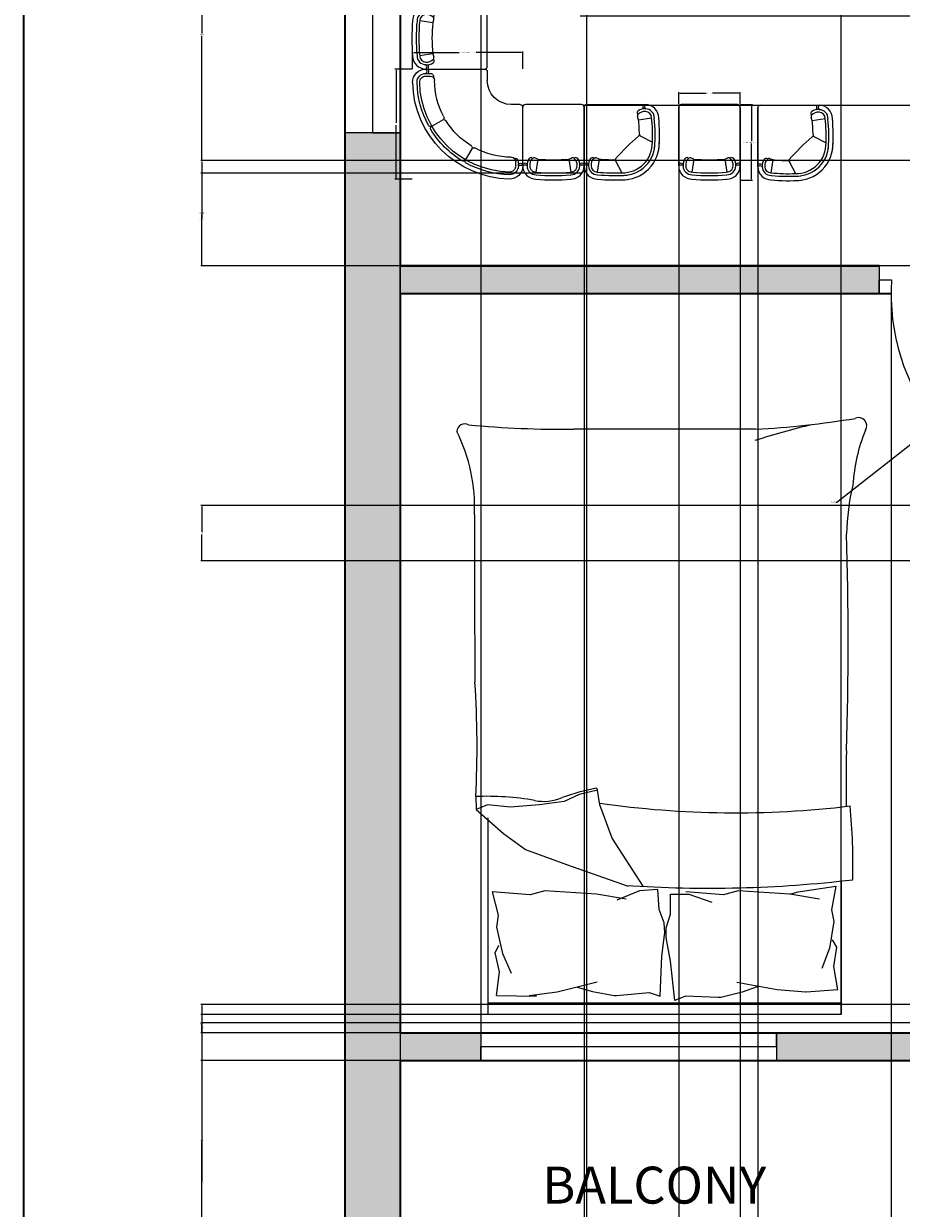
# Model space of a CAD drawing. Units: inches. Extents: x 2606 to 3027, y 1906 to 2463.
# Tile 2 of 10: x 2606 to 2748, y 2004 to 2196. Entities that reach past the tile are written whole.
import ezdxf

# ---------------------------------------------------------------- set-up
doc = ezdxf.new("R2010")
doc.units = ezdxf.units.IN
for name, color, linetype, lineweight in [('A-ANNO-DIMS', 2, 'Continuous', 18), ('A-ANNO-TTLB', 7, 'Continuous', 35), ('A-AREA-IDEN', 7, 'Continuous', 18), ('A-DOOR', 3, 'Continuous', 18), ('A-FURN', 8, 'Continuous', 13), ('A-GLAZ', 4, 'Continuous', 18), ('A-WALL', 7, 'Continuous', 35)]:
    doc.layers.add(name, color=color, linetype=linetype, lineweight=lineweight)
doc.layers.add('A-WALL-PATT', color=251, linetype='Continuous', lineweight=13, true_color=0x636466)
doc.styles.get("Standard").update_dxf_attribs({"font": 'arial.ttf'})
doc.dimstyles.get("Standard").update_dxf_attribs({"dimtxt": 0.18, "dimasz": 0.18, "dimexe": 0.18, "dimexo": 0.0625, "dimgap": 0.09, "dimtad": 0, "dimtih": 1, "dimtoh": 1, "dimdec": 4, "dimzin": 0, "dimdsep": 46, "dimtxsty": 'Standard', "dimcen": 0.09, "dimadec": 0, "dimazin": 0, "dimtfac": 1, "dimtdec": 4, "dimtofl": 0, "dimtmove": 0, "dimatfit": 3, "dimfxl": 1, "dimtolj": 1, "dimtzin": 0, "dimarcsym": 0})

# ---------------------------------------------------------------- blocks, each defined once
blk = doc.blocks.new('A$C707258B2')
at = {"color": 0}
for p, q in [((0.404, 0.342), (1.074, 0.342)), ((0.404, 0.292), (0.454, 0.292)), ((1.104, 0.312), (1.104, 0.212)), ((0.404, 0.262), (0.454, 0.262)), ((1.479, -0.063), (1.379, -0.063)), ((1.509, -0.763), (1.509, -0.093)), ((0.6, -0.238), (0.47, -0.313)), ((0.929, -0.567), (0.854, -0.697)), ((1.429, -0.763), (1.429, -0.713)), ((1.459, -0.763), (1.459, -0.712))]:
    blk.add_line(p, q, dxfattribs=at)
for centre, radius, start, end in [((0.404, 0.192), 0.15, 90, 181.1754), ((0.404, 0.192), 0.1, 90, 181.1754), ((0.378, 0.317), 0.0362, 316.3972, 43.6028), ((0.368, 0.317), 0.0662, 337.8298, 22.1702), ((0.455, 0.256), 0.0357, 345.4262, 90.5555), ((1.074, 0.312), 0.03, 360, 90), ((1.379, 0.212), 1.125, 181.1754, 268.8246), ((1.379, 0.212), 1.075, 181.1754, 208.6357), ((0.404, 0.192), 0.07, 90, 181.1754), ((1.379, 0.212), 1.045, 181.1754, 268.8246), ((0.454, 0.212), 0.05, 360, 90), ((1.379, 0.212), 0.875, 180, 208.4082), ((1.379, 0.212), 0.275, 180, 270), ((1.479, -0.093), 0.03, 360, 90), ((0.587, -0.216), 0.025, 300, 28.4082), ((0.612, -0.259), 0.025, 31.5918, 120), ((1.379, 0.212), 0.875, 211.5918, 238.4082), ((0.457, -0.291), 0.025, 208.6357, 300), ((0.482, -0.334), 0.025, 120, 211.3643), ((1.379, 0.212), 1.075, 211.3643, 238.6357), ((0.907, -0.555), 0.025, 330, 58.4082), ((0.951, -0.58), 0.025, 61.5918, 150), ((1.379, 0.212), 0.875, 241.5918, 270), ((1.379, -0.713), 0.05, 360, 90), ((0.832, -0.685), 0.025, 238.6357, 330), ((0.876, -0.71), 0.025, 150, 241.3643), ((1.379, 0.212), 1.075, 241.3643, 268.8246), ((1.359, -0.763), 0.15, 268.8246, 360), ((1.359, -0.763), 0.1, 268.8246, 360), ((1.359, -0.763), 0.07, 268.8246, 360), ((1.425, -0.709), 0.0336, 354.6301, 109.3883), ((1.484, -0.799), 0.0662, 67.8298, 112.1702), ((1.484, -0.789), 0.0362, 46.3972, 133.6028)]:
    blk.add_arc(centre, radius, start, end, dxfattribs=at)
blk = doc.blocks.new('part 01')
at = {"color": 0}
for p, q in [((-670, 700), (0, 700)), ((-591, 527), (-740, 550)), ((-591, 527), (-579, 561)), ((30, 30), (30, 670)), ((-591, 173), (-740, 150)), ((-591, 173), (-579, 139)), ((-670, 0), (0, 0))]:
    blk.add_line(p, q, dxfattribs=at)
for centre, radius, start, end in [((-670, 550), 150, 90, 181.1754), ((-696, 675), 36.2, 316.3972, 43.6028), ((-706, 675), 66.2, 337.8298, 22.1702), ((0, 670), 30, 0, 90), ((1178, 350), 2008, 174.2835, 185.7165), ((1178, 350), 1958, 174.2835, 185.7165), ((-670, 550), 100, 90, 181.1754), ((1178, 350), 1928, 174.2835, 185.7165), ((-670, 550), 70, 90, 181.1754), ((-660, 518), 133, 56.0897, 95.6132), ((-660, 518), 103, 42.0066, 95.6132), ((-600, 607), 25, 332.9608, 56.0897), ((-625, 620), 53.2, 321.0017, 332.9608), ((-602, 570), 25, 340, 42.0066), ((1178, 350), 1778, 174.2835, 185.7165), ((-670, 150), 150, 178.8246, 270), ((-670, 150), 100, 178.8246, 270), ((-670, 150), 70, 178.8246, 270), ((-602, 130), 25, 317.9934, 20), ((-660, 182), 133, 264.3868, 303.9103), ((-660, 182), 103, 264.3868, 317.9934), ((-696, 25), 36.2, 316.3972, 43.6028), ((-706, 25), 66.2, 337.8298, 22.1702), ((-600, 93), 25, 303.9103, 27.0392), ((-625, 80), 53.2, 27.0392, 38.9983), ((0, 30), 30, 270, 0)]:
    blk.add_arc(centre, radius, start, end, dxfattribs=at)
blk = doc.blocks.new('part02')
at = {"color": 0}
for p, q in [((0, -670), (0, 0)), ((30, 30), (700, 30)), ((621, -143), (609, -109)), ((621, -143), (770, -120)), ((640, -326), (778, -399)), ((173, -591), (139, -579)), ((173, -591), (150, -740)), ((356, -610), (429, -748))]:
    blk.add_line(p, q, dxfattribs=at)
for centre, radius, start, end in [((30, 0), 30, 90, 180), ((726, 5), 56.2, 153.6122, 206.6666), ((726, 5), 36.2, 136.3972, 223.6028), ((700, -120), 150, 0, 90), ((630, -63), 25, 123.9103, 207.0392), ((655, -50), 53.2, 207.0392, 218.9983), ((632, -100), 25, 137.9934, 200), ((690, -152), 103, 84.3868, 137.9934), ((689, -151), 132, 85.4378, 123.9887), ((700, -121), 101, 357.5006, 89.858), ((700, -120), 70, 0, 90), ((-1228, -320), 2008, 357.7349, 5.7032), ((-1148, -320), 1958, 355.8657, 5.7165), ((-1148, -320), 2008, 355.818, 5.7165), ((-1148, -320), 1778, 0.3836, 5.7165), ((2220, -2190), 2454, 130.6961, 139.3039), ((439, -409), 419, 268.2181, 1.7819), ((439, -409), 369, 268.2181, 1.7819), ((439, -409), 339, 268.2181, 1.7819), ((632, -344), 20, 62, 130.6961), ((650, -308), 20, 180.3836, 242), ((25, -696), 56.2, 63.3334, 116.3878), ((25, -696), 36.2, 46.3972, 133.6028), ((150, -670), 150, 180, 271.1754), ((182, -660), 133, 146.0897, 185.6132), ((150, -670), 100, 180, 271.1754), ((93, -600), 25, 62.9608, 146.0897), ((182, -660), 103, 132.0066, 185.6132), ((150, -670), 70, 180, 270), ((80, -625), 53.2, 51.0017, 62.9608), ((130, -602), 25, 70, 132.0066), ((350, 1178), 1778, 264.2835, 269.6164), ((338, -620), 20, 28, 89.6164), ((374, -602), 20, 139.3039, 208), ((350, 1258), 2008, 264.2968, 272.2651), ((350, 1178), 1958, 264.2835, 274.1343), ((350, 1178), 2008, 264.2835, 274.182)]:
    blk.add_arc(centre, radius, start, end, dxfattribs=at)
blk = doc.blocks.new('BED-DOUBLE')
for p, q in [((4.17, 75.16), (4.17, 96.87)), ((4.17, 96.87), (61.46, 96.87)), ((61.46, 96.87), (61.46, 64.97)), ((4.17, 95.03), (61.46, 95.03)), ((29.42, 93.94), (31.15, 94.63)), ((31.15, 94.63), (31.84, 88.22)), ((4.67, 92.87), (9.81, 93.27)), ((4.67, 92.9), (5.36, 89.08)), ((9.81, 93.27), (9.93, 93.24)), ((9.93, 93.24), (14.52, 92.9)), ((14.52, 92.9), (21.1, 91.68)), ((17.81, 92.38), (20.24, 93.24)), ((20.24, 93.24), (23.7, 94.11)), ((23.7, 94.11), (24.09, 94.11)), ((24.09, 94.11), (29.42, 93.94)), ((33.54, 93.89), (33.25, 87.44)), ((35.31, 93.3), (33.54, 93.89)), ((40.62, 93.81), (35.31, 93.3)), ((41.01, 93.83), (40.62, 93.81)), ((44.52, 93.18), (41.01, 93.83)), ((50.25, 93.19), (43.75, 91.57)), ((47, 92.47), (44.52, 93.18)), ((54.8, 93.82), (50.25, 93.19)), ((60.08, 93.81), (53.6, 93.92)), ((53.6, 93.92), (54.8, 93.82)), ((60.08, 93.81), (59.62, 89.96)), ((5.36, 89.08), (4.84, 85.96)), ((6.06, 86.14), (7.27, 89.43)), ((59.12, 86.97), (57.7, 90.18)), ((59.62, 89.96), (60.34, 86.88)), ((31.84, 88.22), (32.54, 84.4)), ((33.25, 87.44), (32.79, 83.59)), ((60.08, 82.69), (59.12, 86.97)), ((60.34, 86.88), (59.72, 85.62)), ((4.84, 85.96), (5.54, 84.75)), ((5.36, 81.8), (6.06, 86.14)), ((32.54, 82.84), (31.84, 80.59)), ((32.54, 84.4), (32.54, 82.84)), ((32.79, 83.59), (32.89, 82.03)), ((5.71, 79.9), (5.36, 81.8)), ((32.89, 82.03), (33.72, 79.83)), ((59.85, 80.77), (60.08, 82.69)), ((5.02, 76.08), (5.71, 79.9)), ((31.84, 80.59), (31.84, 77.38)), ((33.72, 79.83), (33.92, 76.62)), ((60.78, 77), (59.85, 80.77)), ((11.13, 76.95), (5.02, 76.08)), ((7.65, 78.14), (12.48, 77.34)), ((12.48, 77.34), (11.13, 76.95)), ((12.48, 77.34), (20.89, 76.82)), ((20.89, 76.82), (23.24, 77.49)), ((23.24, 77.49), (29.39, 77)), ((28.9, 77.38), (25.13, 78.68)), ((31.84, 77.38), (28.9, 77.38)), ((36.87, 76.8), (40.55, 78.34)), ((39.04, 78.14), (43.87, 77.34)), ((43.87, 77.34), (52.28, 76.82)), ((52.28, 76.82), (54.63, 77.49)), ((54.63, 77.49), (60.78, 77)), ((33.92, 76.62), (36.87, 76.8)), ((36.28, 76.03), (41.3, 68.25)), ((48.73, 72.52), (38.73, 76.03)), ((55.41, 70.1), (48.73, 72.52)), ((58.94, 67.51), (55.41, 70.1)), ((41.3, 68.25), (43.34, 62.87)), ((63.38, 63.61), (58.94, 67.51)), ((61.54, 62.87), (63.38, 63.61)), ((63.48, 61.52), (63.38, 63.61, 4.64)), ((43.34, 62.87), (43.71, 60.45)), ((46.68, 61.2), (49.1, 62.31)), ((49.1, 62.31), (53.18, 62.87)), ((53.18, 62.87), (57.82, 63.24)), ((57.82, 63.24), (61.54, 62.87)), ((43.71, 60.45), (46.68, 61.2)), ((18.06, 1.87), (47.57, 1.87))]:
    blk.add_line(p, q)
for centre, radius, start, end in [((102.1, 72.78), 99.87, 178.7218, 185.604), ((25.61, -121.38), 197.77, 86.0865, 96.7821), ((21.29, -90.53), 154.68, 81.7845, 96.9006), ((-200.58, 59.5), 203.94, 358.4762, 1.0082), ((37.35, 95.1), 35.55, 280.6617, 289.8806), ((52.44, 54.83), 7.46, 78.6608, 113.7384), ((61.53, 104.85), 43.38, 259.8763, 272.5657), ((43.92, 60.38), 0.221, 160.2464, 271.1377), ((218.51, 53.34), 155.25, 176.9791, 183.8365), ((581.23, 36.19), 578.22, 178.22771, 181.71854), ((-5405.34, 15.56), 5469.02, 0.00217, 0.28689), ((-32.25, 19.53), 35.53, 346.0648, 358.9113), ((91.3, 14.55), 27.65, 177.4714, 206.4681), ((-25.97, 12.62), 28.25, 337.9751, 356.652), ((1.3, 1.3), 1.31, 146.1736, 293.4781), ((-20.65, 125.3), 127.63, 283.3832, 287.7053), ((65.23, 2.32), 1.32, 242.6588, 356.02), ((25.69, -143.9), 145.97, 92.9958, 99.4091), ((49.34, -157.62), 159.5, 84.4998, 90.6351)]:
    blk.add_arc(centre, radius, start, end)
blk = doc.blocks.new('WIN-60IN')
for p, q in [((0, 9), (0, 0)), ((60, 4.5), (60, 9)), ((60, 9), (60, 0)), ((0, 0), (0, 4.5)), ((0, 4.5), (60, 4.5))]:
    blk.add_line(p, q)
blk = doc.blocks.new('WIN-48IN')
for p, q in [((0, 4.5), (0, 0)), ((48, 2.25), (48, 4.5)), ((48, 4.5), (48, 0)), ((0, 0), (0, 2.25)), ((0, 2.25), (48, 2.25))]:
    blk.add_line(p, q)
blk = doc.blocks.new('*D17')
at = {"layer": 'A-ANNO-DIMS', "color": 0, "lineweight": -2, "transparency": 16777216}
for p, q in [((2722.29, 2183.31), (2724.25, 2183.31)), ((2724.07, 2183.13), (2724.07, 2177.34)), ((2724.07, 2171.2), (2724.07, 2176.98)), ((2722.29, 2171.02), (2724.25, 2171.02))]:
    blk.add_line(p, q, dxfattribs=at)
at = {"layer": 'A-ANNO-DIMS', "color": 0, "transparency": 16777216}
for points in [[(2724.04, 2183.13), (2724.1, 2183.13), (2724.07, 2183.31)], [(2724.04, 2171.2), (2724.1, 2171.2), (2724.07, 2171.02)]]:
    blk.add_solid(points, dxfattribs=at)
at = {"layer": 'Defpoints', "color": 0, "transparency": 16777216}
for p in [(2722.23, 2183.31), (2724.07, 2183.31), (2722.23, 2171.02)]:
    blk.add_point(p, dxfattribs=at)
at = {"layer": 'A-ANNO-DIMS', "color": 0, "transparency": 16777216, "insert": (2724.07, 2177.16), "char_height": 0.18, "attachment_point": 5}
blk.add_mtext('\\A1;SEAT MODULE 12 TYP.', dxfattribs=at)
blk = doc.blocks.new('*D18')
at = {"layer": 'A-ANNO-DIMS', "color": 0, "lineweight": -2, "transparency": 16777216}
for p, q in [((2712.26, 2183.37), (2712.26, 2185.33)), ((2712.44, 2185.15), (2716.72, 2185.15)), ((2722.05, 2185.15), (2717.76, 2185.15)), ((2722.23, 2183.37), (2722.23, 2185.33))]:
    blk.add_line(p, q, dxfattribs=at)
at = {"layer": 'A-ANNO-DIMS', "color": 0, "transparency": 16777216}
for points in [[(2712.44, 2185.18), (2712.44, 2185.12), (2712.26, 2185.15)], [(2722.05, 2185.18), (2722.05, 2185.12), (2722.23, 2185.15)]]:
    blk.add_solid(points, dxfattribs=at)
at = {"layer": 'Defpoints', "color": 0, "transparency": 16777216}
for p in [(2712.26, 2185.15), (2712.26, 2183.31), (2722.23, 2183.31)]:
    blk.add_point(p, dxfattribs=at)
at = {"layer": 'A-ANNO-DIMS', "color": 0, "transparency": 16777216, "insert": (2717.24, 2185.15), "char_height": 0.18, "attachment_point": 5}
blk.add_mtext('\\A1;10 TYP.', dxfattribs=at)
blk = doc.blocks.new('*D21')
at = {"layer": 'A-ANNO-DIMS', "color": 0, "lineweight": -2, "transparency": 16777216}
for p, q in [((2669.06, 2189.13), (2669.06, 2191.93)), ((2669.24, 2191.75), (2676.63, 2191.75)), ((2686.76, 2191.75), (2679.37, 2191.75)), ((2686.94, 2189.13), (2686.94, 2191.93))]:
    blk.add_line(p, q, dxfattribs=at)
at = {"layer": 'A-ANNO-DIMS', "color": 0, "transparency": 16777216}
for points in [[(2669.24, 2191.78), (2669.24, 2191.72), (2669.06, 2191.75)], [(2686.76, 2191.78), (2686.76, 2191.72), (2686.94, 2191.75)]]:
    blk.add_solid(points, dxfattribs=at)
at = {"layer": 'Defpoints', "color": 0, "transparency": 16777216}
for p in [(2686.94, 2191.75), (2669.06, 2189.07), (2686.94, 2189.07)]:
    blk.add_point(p, dxfattribs=at)
at = {"layer": 'A-ANNO-DIMS', "color": 0, "transparency": 16777216, "insert": (2678, 2191.75), "char_height": 0.18, "attachment_point": 5}
blk.add_mtext('\\A1;CORNER MODULE 18', dxfattribs=at)
blk = doc.blocks.new('*D22')
at = {"layer": 'A-ANNO-DIMS', "color": 0, "lineweight": -2, "transparency": 16777216}
for p, q in [((2669, 2189.07), (2666.2, 2189.07)), ((2666.38, 2188.89), (2666.38, 2180.31)), ((2666.38, 2171.37), (2666.38, 2179.95)), ((2669, 2171.19), (2666.2, 2171.19))]:
    blk.add_line(p, q, dxfattribs=at)
at = {"layer": 'A-ANNO-DIMS', "color": 0, "transparency": 16777216}
for points in [[(2666.35, 2188.89), (2666.41, 2188.89), (2666.38, 2189.07)], [(2666.35, 2171.37), (2666.41, 2171.37), (2666.38, 2171.19)]]:
    blk.add_solid(points, dxfattribs=at)
at = {"layer": 'Defpoints', "color": 0, "transparency": 16777216}
for p in [(2666.38, 2189.07), (2669.06, 2189.07), (2669.06, 2171.19)]:
    blk.add_point(p, dxfattribs=at)
at = {"layer": 'A-ANNO-DIMS', "color": 0, "transparency": 16777216, "insert": (2666.38, 2180.13), "char_height": 0.18, "attachment_point": 5}
blk.add_mtext('\\A1;18', dxfattribs=at)
blk = doc.blocks.new('*D32')
at = {"layer": 'A-ANNO-DIMS', "color": 0, "lineweight": -2, "transparency": 16777216}
for p, q in [((2667.06, 2032.67), (2667.06, 2433.99)), ((2667.24, 2433.81), (2673.16, 2433.81)), ((2679.99, 2433.81), (2674.07, 2433.81)), ((2680.17, 2032.67), (2680.17, 2433.99))]:
    blk.add_line(p, q, dxfattribs=at)
at = {"layer": 'A-ANNO-DIMS', "color": 0, "transparency": 16777216}
for points in [[(2667.24, 2433.84), (2667.24, 2433.78), (2667.06, 2433.81)], [(2679.99, 2433.84), (2679.99, 2433.78), (2680.17, 2433.81)]]:
    blk.add_solid(points, dxfattribs=at)
at = {"layer": 'Defpoints', "color": 0, "transparency": 16777216}
for p in [(2680.17, 2433.81), (2667.06, 2032.61), (2680.17, 2032.61)]:
    blk.add_point(p, dxfattribs=at)
at = {"layer": 'A-ANNO-DIMS', "color": 0, "transparency": 16777216, "insert": (2673.61, 2433.81), "char_height": 0.18, "attachment_point": 5}
blk.add_mtext('\\A1;13.102', dxfattribs=at)
blk = doc.blocks.new('*D37')
at = {"layer": 'A-ANNO-DIMS', "color": 0, "lineweight": -2, "transparency": 16777216}
for p, q in [((2667, 2028.11), (2634.68, 2028.11)), ((2634.86, 2027.93), (2634.86, 2008.54)), ((2634.86, 1988.79), (2634.86, 2008.18)), ((2658, 1988.61), (2634.68, 1988.61))]:
    blk.add_line(p, q, dxfattribs=at)
at = {"layer": 'A-ANNO-DIMS', "color": 0, "transparency": 16777216}
for points in [[(2634.83, 2027.93), (2634.89, 2027.93), (2634.86, 2028.11)], [(2634.83, 1988.79), (2634.89, 1988.79), (2634.86, 1988.61)]]:
    blk.add_solid(points, dxfattribs=at)
at = {"layer": 'Defpoints', "color": 0, "transparency": 16777216}
for p in [(2634.86, 2028.11), (2667.06, 2028.11), (2658.06, 1988.61)]:
    blk.add_point(p, dxfattribs=at)
at = {"layer": 'A-ANNO-DIMS', "color": 0, "transparency": 16777216, "insert": (2634.86, 2008.36), "char_height": 0.18, "attachment_point": 5}
blk.add_mtext('\\A1;39.5', dxfattribs=at)
blk = doc.blocks.new('*D39')
at = {"layer": 'A-ANNO-DIMS', "color": 0, "lineweight": -2, "transparency": 16777216}
for p, q in [((2847.5, 2118.21), (2634.68, 2118.21)), ((2634.86, 2118.03), (2634.86, 2113.89)), ((2634.86, 2109.39), (2634.86, 2113.53)), ((2847.5, 2109.21), (2634.68, 2109.21))]:
    blk.add_line(p, q, dxfattribs=at)
at = {"layer": 'A-ANNO-DIMS', "color": 0, "transparency": 16777216}
for points in [[(2634.83, 2118.03), (2634.89, 2118.03), (2634.86, 2118.21)], [(2634.83, 2109.39), (2634.89, 2109.39), (2634.86, 2109.21)]]:
    blk.add_solid(points, dxfattribs=at)
at = {"layer": 'Defpoints', "color": 0, "transparency": 16777216}
for p in [(2847.56, 2118.21), (2634.86, 2109.21), (2847.56, 2109.21)]:
    blk.add_point(p, dxfattribs=at)
at = {"layer": 'A-ANNO-DIMS', "color": 0, "transparency": 16777216, "insert": (2634.86, 2113.71), "char_height": 0.18, "attachment_point": 5}
blk.add_mtext('\\A1;9', dxfattribs=at)
blk = doc.blocks.new('*D40')
at = {"layer": 'A-ANNO-DIMS', "color": 0, "lineweight": -2, "transparency": 16777216}
for p, q in [((2847.5, 2037.21), (2634.68, 2037.21)), ((2634.86, 2037.03), (2634.86, 2015.34)), ((2634.86, 1993.29), (2634.86, 2014.98)), ((2847.5, 1993.11), (2634.68, 1993.11))]:
    blk.add_line(p, q, dxfattribs=at)
at = {"layer": 'A-ANNO-DIMS', "color": 0, "transparency": 16777216}
for points in [[(2634.83, 2037.03), (2634.89, 2037.03), (2634.86, 2037.21)], [(2634.83, 1993.29), (2634.89, 1993.29), (2634.86, 1993.11)]]:
    blk.add_solid(points, dxfattribs=at)
at = {"layer": 'Defpoints', "color": 0, "transparency": 16777216}
for p in [(2847.56, 2037.21), (2634.86, 1993.11), (2847.56, 1993.11)]:
    blk.add_point(p, dxfattribs=at)
at = {"layer": 'A-ANNO-DIMS', "color": 0, "transparency": 16777216, "insert": (2634.86, 2015.16), "char_height": 0.18, "attachment_point": 5}
blk.add_mtext('\\A1;44.1', dxfattribs=at)
blk = doc.blocks.new('*D45')
at = {"layer": 'A-ANNO-DIMS', "color": 0, "lineweight": -2, "transparency": 16777216}
for p, q in [((2746.75, 2152.55), (2746.75, 1965.23)), ((2775.13, 2152.55), (2775.13, 1965.23)), ((2746.93, 1965.41), (2760.47, 1965.41)), ((2774.95, 1965.41), (2761.4, 1965.41))]:
    blk.add_line(p, q, dxfattribs=at)
at = {"layer": 'A-ANNO-DIMS', "color": 0, "transparency": 16777216}
for points in [[(2746.93, 1965.44), (2746.93, 1965.38), (2746.75, 1965.41)], [(2774.95, 1965.44), (2774.95, 1965.38), (2775.13, 1965.41)]]:
    blk.add_solid(points, dxfattribs=at)
at = {"layer": 'Defpoints', "color": 0, "transparency": 16777216}
for p in [(2746.75, 2152.61), (2775.13, 2152.61), (2775.13, 1965.41)]:
    blk.add_point(p, dxfattribs=at)
at = {"layer": 'A-ANNO-DIMS', "color": 0, "transparency": 16777216, "insert": (2760.94, 1965.41), "char_height": 0.18, "attachment_point": 5}
blk.add_mtext('\\A1;28.384', dxfattribs=at)
blk = doc.blocks.new('*D61')
at = {"layer": 'A-ANNO-DIMS', "color": 0, "lineweight": -2, "transparency": 16777216}
for p, q in [((2696.29, 2197.72), (3000.44, 2197.72)), ((3000.26, 2197.54), (3000.26, 2190.63)), ((3000.26, 2183.36), (3000.26, 2190.27)), ((2696.84, 2183.18), (3000.44, 2183.18))]:
    blk.add_line(p, q, dxfattribs=at)
at = {"layer": 'A-ANNO-DIMS', "color": 0, "transparency": 16777216}
for points in [[(3000.23, 2197.54), (3000.29, 2197.54), (3000.26, 2197.72)], [(3000.23, 2183.36), (3000.29, 2183.36), (3000.26, 2183.18)]]:
    blk.add_solid(points, dxfattribs=at)
at = {"layer": 'Defpoints', "color": 0, "transparency": 16777216}
for p in [(2696.23, 2197.72), (3000.26, 2197.72), (2696.78, 2183.18)]:
    blk.add_point(p, dxfattribs=at)
at = {"layer": 'A-ANNO-DIMS', "color": 0, "transparency": 16777216, "insert": (3000.26, 2190.45), "char_height": 0.18, "attachment_point": 5}
blk.add_mtext('\\A1;14.545', dxfattribs=at)
blk = doc.blocks.new('*D62')
at = {"layer": 'A-ANNO-DIMS', "color": 0, "lineweight": -2, "transparency": 16777216}
for p, q in [((2696.48, 2172.14), (2634.68, 2172.14)), ((2634.86, 2171.96), (2634.86, 2164.81)), ((2634.86, 2157.29), (2634.86, 2164.44)), ((2667, 2157.11), (2634.68, 2157.11))]:
    blk.add_line(p, q, dxfattribs=at)
at = {"layer": 'A-ANNO-DIMS', "color": 0, "transparency": 16777216}
for points in [[(2634.83, 2171.96), (2634.89, 2171.96), (2634.86, 2172.14)], [(2634.83, 2157.29), (2634.89, 2157.29), (2634.86, 2157.11)]]:
    blk.add_solid(points, dxfattribs=at)
at = {"layer": 'Defpoints', "color": 0, "transparency": 16777216}
for p in [(2634.86, 2172.14), (2696.54, 2172.14), (2667.06, 2157.11)]:
    blk.add_point(p, dxfattribs=at)
at = {"layer": 'A-ANNO-DIMS', "color": 0, "transparency": 16777216, "insert": (2634.86, 2164.63), "char_height": 0.18, "attachment_point": 5}
blk.add_mtext('\\A1;15.033', dxfattribs=at)
blk = doc.blocks.new('*D64')
at = {"layer": 'A-ANNO-DIMS', "color": 0, "lineweight": -2, "transparency": 16777216}
for p, q in [((2696.91, 2182.82), (2696.91, 1965.23)), ((2712.26, 2182.82), (2712.26, 1965.23)), ((2697.09, 1965.41), (2704.13, 1965.41)), ((2712.08, 1965.41), (2705.04, 1965.41))]:
    blk.add_line(p, q, dxfattribs=at)
at = {"layer": 'A-ANNO-DIMS', "color": 0, "transparency": 16777216}
for points in [[(2697.09, 1965.44), (2697.09, 1965.38), (2696.91, 1965.41)], [(2712.08, 1965.44), (2712.08, 1965.38), (2712.26, 1965.41)]]:
    blk.add_solid(points, dxfattribs=at)
at = {"layer": 'Defpoints', "color": 0, "transparency": 16777216}
for p in [(2696.91, 2182.88), (2712.26, 2182.88), (2712.26, 1965.41)]:
    blk.add_point(p, dxfattribs=at)
at = {"layer": 'A-ANNO-DIMS', "color": 0, "transparency": 16777216, "insert": (2704.58, 1965.41), "char_height": 0.18, "attachment_point": 5}
blk.add_mtext('\\A1;15.354', dxfattribs=at)
blk = doc.blocks.new('*D65')
at = {"layer": 'A-ANNO-DIMS', "color": 0, "lineweight": -2, "transparency": 16777216}
for p, q in [((2722.23, 2182.82), (2722.23, 1965.23)), ((2725.1, 2182.7), (2725.1, 1965.23)), ((2722.41, 1965.41), (2723.34, 1965.41)), ((2724.92, 1965.41), (2723.99, 1965.41))]:
    blk.add_line(p, q, dxfattribs=at)
at = {"layer": 'A-ANNO-DIMS', "color": 0, "transparency": 16777216}
for points in [[(2722.41, 1965.44), (2722.41, 1965.38), (2722.23, 1965.41)], [(2724.92, 1965.44), (2724.92, 1965.38), (2725.1, 1965.41)]]:
    blk.add_solid(points, dxfattribs=at)
at = {"layer": 'Defpoints', "color": 0, "transparency": 16777216}
for p in [(2722.23, 2182.88), (2725.1, 2182.76), (2725.1, 1965.41)]:
    blk.add_point(p, dxfattribs=at)
at = {"layer": 'A-ANNO-DIMS', "color": 0, "transparency": 16777216, "insert": (2723.66, 1965.41), "char_height": 0.18, "attachment_point": 5}
blk.add_mtext('\\A1;2.87', dxfattribs=at)
blk = doc.blocks.new('*D68')
at = {"layer": 'A-ANNO-DIMS', "color": 0, "lineweight": -2, "transparency": 16777216}
for p, q in [((2897, 2215.13), (2634.68, 2215.13)), ((2634.86, 2214.95), (2634.86, 2194.85)), ((2634.86, 2174.38), (2634.86, 2194.48)), ((2897, 2174.2), (2634.68, 2174.2))]:
    blk.add_line(p, q, dxfattribs=at)
at = {"layer": 'A-ANNO-DIMS', "color": 0, "transparency": 16777216}
for points in [[(2634.83, 2214.95), (2634.89, 2214.95), (2634.86, 2215.13)], [(2634.83, 2174.38), (2634.89, 2174.38), (2634.86, 2174.2)]]:
    blk.add_solid(points, dxfattribs=at)
at = {"layer": 'Defpoints', "color": 0, "transparency": 16777216}
for p in [(2897.06, 2215.13), (2634.86, 2174.2), (2897.06, 2174.2)]:
    blk.add_point(p, dxfattribs=at)
at = {"layer": 'A-ANNO-DIMS', "color": 0, "transparency": 16777216, "insert": (2634.86, 2194.66), "char_height": 0.18, "attachment_point": 5}
blk.add_mtext('\\A1;40.94', dxfattribs=at)
blk = doc.blocks.new('*D69')
at = {"layer": 'A-ANNO-DIMS', "color": 0, "lineweight": -2, "transparency": 16777216}
for p, q in [((2897, 2174.2), (2634.68, 2174.2)), ((2634.86, 2174.02), (2634.86, 2165.84)), ((2634.86, 2157.29), (2634.86, 2165.47)), ((2897, 2157.11), (2634.68, 2157.11))]:
    blk.add_line(p, q, dxfattribs=at)
at = {"layer": 'A-ANNO-DIMS', "color": 0, "transparency": 16777216}
for points in [[(2634.83, 2174.02), (2634.89, 2174.02), (2634.86, 2174.2)], [(2634.83, 2157.29), (2634.89, 2157.29), (2634.86, 2157.11)]]:
    blk.add_solid(points, dxfattribs=at)
at = {"layer": 'Defpoints', "color": 0, "transparency": 16777216}
for p in [(2897.06, 2174.2), (2634.86, 2157.11), (2897.06, 2157.11)]:
    blk.add_point(p, dxfattribs=at)
at = {"layer": 'A-ANNO-DIMS', "color": 0, "transparency": 16777216, "insert": (2634.86, 2165.65), "char_height": 0.18, "attachment_point": 5}
blk.add_mtext('\\A1;17.087', dxfattribs=at)
blk = doc.blocks.new('*D74')
at = {"layer": 'A-ANNO-DIMS', "color": 0, "lineweight": -2, "transparency": 16777216}
for p, q in [((2667.06, 2401.55), (2667.06, 1965.23)), ((2697.29, 2399.09), (2697.29, 1965.23)), ((2667.24, 1965.41), (2681.71, 1965.41)), ((2697.11, 1965.41), (2682.64, 1965.41))]:
    blk.add_line(p, q, dxfattribs=at)
at = {"layer": 'A-ANNO-DIMS', "color": 0, "transparency": 16777216}
for points in [[(2667.24, 1965.44), (2667.24, 1965.38), (2667.06, 1965.41)], [(2697.11, 1965.44), (2697.11, 1965.38), (2697.29, 1965.41)]]:
    blk.add_solid(points, dxfattribs=at)
at = {"layer": 'Defpoints', "color": 0, "transparency": 16777216}
for p in [(2667.06, 2401.61), (2697.29, 2399.15), (2667.06, 1965.41)]:
    blk.add_point(p, dxfattribs=at)
at = {"layer": 'A-ANNO-DIMS', "color": 0, "transparency": 16777216, "insert": (2682.18, 1965.41), "char_height": 0.18, "attachment_point": 5}
blk.add_mtext('\\A1;30.225', dxfattribs=at)
blk = doc.blocks.new('*D76')
at = {"layer": 'A-ANNO-DIMS', "color": 0, "lineweight": -2, "transparency": 16777216}
for p, q in [((2738.62, 2035.66), (2738.62, 2433.99)), ((2738.8, 2433.81), (2760.37, 2433.81)), ((2782.88, 2433.81), (2761.31, 2433.81)), ((2783.06, 2032.67), (2783.06, 2433.99))]:
    blk.add_line(p, q, dxfattribs=at)
at = {"layer": 'A-ANNO-DIMS', "color": 0, "transparency": 16777216}
for points in [[(2738.8, 2433.84), (2738.8, 2433.78), (2738.62, 2433.81)], [(2782.88, 2433.84), (2782.88, 2433.78), (2783.06, 2433.81)]]:
    blk.add_solid(points, dxfattribs=at)
at = {"layer": 'Defpoints', "color": 0, "transparency": 16777216}
for p in [(2783.06, 2433.81), (2738.62, 2035.6), (2783.06, 2032.61)]:
    blk.add_point(p, dxfattribs=at)
at = {"layer": 'A-ANNO-DIMS', "color": 0, "transparency": 16777216, "insert": (2760.84, 2433.81), "char_height": 0.18, "attachment_point": 5}
blk.add_mtext('\\A1;44.445', dxfattribs=at)
blk = doc.blocks.new('*D80')
at = {"layer": 'A-ANNO-DIMS', "color": 0, "lineweight": -2, "transparency": 16777216}
for p, q in [((2681.26, 2035.6), (2634.68, 2035.6)), ((2634.86, 2035.42), (2634.86, 2034.29)), ((2634.86, 2032.79), (2634.86, 2033.92)), ((2680.1, 2032.61), (2634.68, 2032.61))]:
    blk.add_line(p, q, dxfattribs=at)
at = {"layer": 'A-ANNO-DIMS', "color": 0, "transparency": 16777216}
for points in [[(2634.83, 2035.42), (2634.89, 2035.42), (2634.86, 2035.6)], [(2634.83, 2032.79), (2634.89, 2032.79), (2634.86, 2032.61)]]:
    blk.add_solid(points, dxfattribs=at)
at = {"layer": 'Defpoints', "color": 0, "transparency": 16777216}
for p in [(2681.32, 2035.6), (2634.86, 2032.61), (2680.17, 2032.61)]:
    blk.add_point(p, dxfattribs=at)
at = {"layer": 'A-ANNO-DIMS', "color": 0, "transparency": 16777216, "insert": (2634.86, 2034.1), "char_height": 0.18, "attachment_point": 5}
blk.add_mtext('\\A1;2.988', dxfattribs=at)
blk = doc.blocks.new('*D81')
at = {"layer": 'A-ANNO-DIMS', "color": 0, "lineweight": -2, "transparency": 16777216}
for p, q in [((2961.6, 2034.23), (2634.68, 2034.23)), ((2634.86, 2034.05), (2634.86, 2033.6)), ((2634.86, 2032.79), (2634.86, 2033.24)), ((2950.83, 2032.61), (2634.68, 2032.61))]:
    blk.add_line(p, q, dxfattribs=at)
at = {"layer": 'A-ANNO-DIMS', "color": 0, "transparency": 16777216}
for points in [[(2634.83, 2034.05), (2634.89, 2034.05), (2634.86, 2034.23)], [(2634.83, 2032.79), (2634.89, 2032.79), (2634.86, 2032.61)]]:
    blk.add_solid(points, dxfattribs=at)
at = {"layer": 'Defpoints', "color": 0, "transparency": 16777216}
for p in [(2961.66, 2034.23), (2634.86, 2032.61), (2950.89, 2032.61)]:
    blk.add_point(p, dxfattribs=at)
at = {"layer": 'A-ANNO-DIMS', "color": 0, "transparency": 16777216, "insert": (2634.86, 2033.42), "char_height": 0.18, "attachment_point": 5}
blk.add_mtext('\\A1;1.62', dxfattribs=at)
blk = doc.blocks.new('*D86')
at = {"layer": 'A-ANNO-DIMS', "color": 0, "lineweight": -2, "transparency": 16777216}
for p, q in [((2780.83, 2152.54), (2781.01, 2152.54)), ((2780.92, 2152.45), (2780.92, 2152.63)), ((2737.93, 2118.74), (2753.91, 2131.31)), ((2737.75, 2118.74), (2737.93, 2118.74))]:
    blk.add_line(p, q, dxfattribs=at)
at = {"layer": 'A-ANNO-DIMS', "color": 0, "transparency": 16777216}
blk.add_solid([(2753.9, 2131.33), (2753.93, 2131.28), (2754.06, 2131.42)], dxfattribs=at)
at = {"layer": 'Defpoints', "color": 0, "transparency": 16777216}
for p in [(2780.92, 2152.54), (2754.06, 2131.42)]:
    blk.add_point(p, dxfattribs=at)
at = {"layer": 'A-ANNO-DIMS', "color": 0, "transparency": 16777216, "insert": (2737.27, 2118.74), "char_height": 0.18, "attachment_point": 5}
blk.add_mtext('\\A1;R34.18', dxfattribs=at)

msp = doc.modelspace()

# ---------------------------------------------------------------- hatches: boundary and pattern name
at = {"layer": 'A-WALL-PATT'}
h = msp.add_hatch(color=256, dxfattribs=at)
h.dxf.hatch_style = 1
h.paths.add_polyline_path([(2667.063, 2401.6097), (2691.9697, 2401.6097), (2691.9697, 2406.1097), (2691.9697, 2410.6097), (2658.063, 2410.6097), (2658.063, 2238.7051), (2667.063, 2238.7051)])
h.paths.add_polyline_path([(2804.9965, 2406.1097), (2804.9965, 2410.6097), (2751.9697, 2410.6097), (2751.9697, 2401.6097), (2783.063, 2401.6097), (2783.063, 2257.6097), (2778.6739, 2257.6097), (2778.6739, 2253.1097), (2792.3386, 2253.1097), (2792.3386, 2255.3597), (2792.3386, 2257.6097), (2787.563, 2257.6097), (2787.563, 2327.1097), (2847.563, 2327.1097), (2847.563, 2331.6097), (2787.563, 2331.6097), (2787.563, 2401.6097), (2804.9965, 2401.6097)])
h.paths.add_polyline_path([(2889.6183, 2406.1097), (2889.6183, 2410.6097), (2828.9965, 2410.6097), (2828.9965, 2401.6097), (2831.8174, 2401.6097), (2847.563, 2401.6097), (2847.563, 2357.8311), (2849.813, 2357.8311), (2852.063, 2357.8311), (2852.063, 2401.6097), (2889.6183, 2401.6097)])
h.paths.add_polyline_path([(2977.063, 2410.6097), (2949.6183, 2410.6097), (2949.6183, 2401.6097), (2968.063, 2401.6097), (2968.063, 2157.1097), (2897.063, 2157.1097), (2897.063, 2174.1966), (2892.563, 2174.1966), (2892.563, 2157.1097), (2886.8122, 2157.1097), (2886.8122, 2152.6097), (2968.063, 2152.6097), (2968.063, 2032.6097), (2950.8911, 2032.6097), (2950.8911, 2028.1097), (2968.063, 2028.1097), (2968.063, 1993.1097), (2852.063, 1993.1097), (2852.063, 2028.1097), (2856.0743, 2028.1097), (2856.0743, 2030.3597), (2856.0743, 2032.6097), (2852.063, 2032.6097), (2852.063, 2152.6097), (2857.369, 2152.6097), (2857.369, 2154.8597), (2857.369, 2157.1097), (2847.563, 2157.1097), (2847.563, 2152.6097), (2847.563, 1993.1097), (2837.0415, 1993.1097), (2837.0415, 1988.6097), (2977.063, 1988.6097)])
h.paths.add_polyline_path([(2968.063, 2257.6097), (2886.9679, 2257.6097), (2886.9679, 2253.1097), (2892.563, 2253.1097), (2892.563, 2215.1332), (2897.063, 2215.1332), (2897.063, 2253.1097), (2968.063, 2253.1097)], flags=17)
h.paths.add_polyline_path([(2856.057, 2255.3597), (2856.057, 2257.6097), (2852.063, 2257.6097), (2852.063, 2336.7476), (2849.813, 2336.7476), (2847.563, 2336.7476), (2847.563, 2331.6097), (2847.563, 2327.1097), (2847.563, 2257.6097), (2813.482, 2257.6097), (2813.482, 2253.1097), (2856.057, 2253.1097)])
h.paths.add_polyline_path([(2748.8874, 2255.3597), (2748.8874, 2257.6097), (2667.063, 2257.6097), (2667.063, 2253.1097), (2748.8874, 2253.1097)])
h.paths.add_polyline_path([(2667.063, 2152.6097), (2744.8238, 2152.6097), (2744.8238, 2154.8597), (2744.8238, 2157.1097), (2667.063, 2157.1097), (2667.063, 2178.7051), (2658.063, 2178.7051), (2658.063, 1988.6097), (2801.0415, 1988.6097), (2801.0415, 1990.8597), (2801.0415, 1993.1097), (2787.563, 1993.1097), (2787.563, 2157.1097), (2777.1295, 2157.1097), (2777.1295, 2152.6097), (2783.063, 2152.6097), (2783.063, 2032.6097), (2778.4484, 2032.6097), (2778.4484, 2028.1097), (2783.063, 2028.1097), (2783.063, 1993.1097), (2667.063, 1993.1097), (2667.063, 2028.1097), (2680.1652, 2028.1097), (2680.1652, 2030.3597), (2680.1652, 2032.6097), (2667.063, 2032.6097)])
h.paths.add_polyline_path([(2755.4074, 2032.6097), (2728.1652, 2032.6097), (2728.1652, 2028.1097), (2755.4074, 2028.1097), (2755.4074, 2030.3597)], flags=17)
h.paths.add_polyline_path([(2902.8911, 2030.3597), (2902.8911, 2032.6097), (2877.6885, 2032.6097), (2877.6885, 2028.1097), (2902.8911, 2028.1097)], flags=17)
h.paths.add_polyline_path([(2810.2211, 2267.221), (2851.2716, 2267.221), (2851.2716, 2289.6098), (2810.2211, 2289.6098)], flags=9)

# ---------------------------------------------------------------- linework, layer by layer
at = {"layer": 'A-ANNO-TTLB'}
msp.add_lwpolyline([(2605.9227, 2462.7868), (3027.4339, 2462.7868), (3027.4339, 1905.5336), (2605.9227, 1905.5336)], close=True, dxfattribs=at)
at = {"layer": 'A-DOOR'}
for p, q in [((2744.8238, 2157.1097), (2744.8238, 2152.6097)), ((2744.8238, 2152.6097), (2744.8238, 2154.8597)), ((2744.8238, 2154.8597), (2746.8238, 2154.8597))]:
    msp.add_line(p, q, dxfattribs=at)
msp.add_arc((2780.9223, 2152.5424), 34.1772, 176.112165, 260.241721, dxfattribs=at)
at = {"layer": 'A-WALL'}
for p, q in [((2658.063, 2410.6097), (2658.063, 1988.6097)), ((2667.063, 2401.6097), (2667.063, 2157.1097)), ((2667.063, 2157.1097), (2744.8238, 2157.1097)), ((2667.063, 2157.1097), (2744.8238, 2157.1097)), ((2744.8238, 2157.1097), (2667.063, 2157.1097)), ((2667.063, 2152.6097), (2746.7452, 2152.6097)), ((2667.063, 2152.6097), (2746.7452, 2152.6097)), ((2667.063, 2152.6097), (2667.063, 2032.6097)), ((2667.063, 2032.6097), (2755.4074, 2032.6097)), ((2667.063, 2028.1097), (2757.5103, 2028.1097)), ((2667.063, 2028.1097), (2667.063, 1993.1097))]:
    msp.add_line(p, q, dxfattribs=at)

# ---------------------------------------------------------------- block references
at = {"layer": 'A-FURN', "ltscale": 0.03, "xscale": 0.0142384057136167, "yscale": 0.0142384057136167, "zscale": 0.0142384057136167}
for name, p in [('part 01', (2680.7465, 2189.0719)), ('part02', (2696.9071, 2182.8782)), ('part02', (2725.1011, 2182.7588))]:
    msp.add_blockref(name, p, dxfattribs=at)
at = {"layer": 'A-FURN', "ltscale": 0.03}
for name, p, xscale, yscale, zscale, rotation in [('A$C707258B2', (2682.0704, 2167.5869), -14.23840571361665, 14.23840571361665, 14.23840571361665, 269.9999999999968), ('part 01', (2696.9071, 2182.8782), 0.0142384057136167, 0.0142384057136167, 0.0142384057136167, 90), ('part 01', (2722.2278, 2182.8782), 0.0142384057136167, 0.0142384057136167, 0.0142384057136167, 90)]:
    msp.add_blockref(name, p, dxfattribs=dict(at, xscale=xscale, yscale=yscale, zscale=zscale, rotation=rotation))
at = {"layer": 'A-FURN', "rotation": 180}
msp.add_blockref('BED-DOUBLE', (2742.7841, 2132.4701), dxfattribs=at)
at = {"layer": 'A-GLAZ', "rotation": 270.0000000000001}
msp.add_blockref('WIN-60IN', (2658.0633, 2238.7048), dxfattribs=at)
at = {"layer": 'A-GLAZ'}
msp.add_blockref('WIN-48IN', (2680.1651, 2028.11), dxfattribs=at)

# ---------------------------------------------------------------- texts
at = {"layer": 'A-AREA-IDEN', "insert": (2690.1075, 2010.8806), "char_height": 6, "attachment_point": 1}
msp.add_mtext_dynamic_manual_height_columns('BALCONY\\P2\'11"', width=32.965259, gutter_width=12.5, heights=[0], dxfattribs=at)

# ---------------------------------------------------------------- dimensions: what is measured, and where the dimension line sits
at = {"layer": 'A-ANNO-DIMS'}
for base, p1, p2, override, picture, middle in [((2680.1652, 2433.8097), (2667.063, 2032.6097), (2680.1652, 2032.6097), {"dimdec": 3, "dimlfac": 1, "dimrnd": 0, "dimzin": 0, "dimdsep": 46, "dimlunit": 2}, '*D32', (2673.6141, 2433.8097)), ((2783.063, 2433.8097), (2738.6178, 2035.5977), (2783.063, 2032.6097), {"dimdec": 3, "dimlfac": 1, "dimrnd": 0, "dimzin": 0, "dimdsep": 46, "dimlunit": 2}, '*D76', (2760.8404, 2433.8097)), ((2667.063, 1965.4097), (2697.2878, 2399.1511), (2667.063, 2401.6097), {"dimdec": 3, "dimlfac": 1, "dimrnd": 0, "dimzin": 0, "dimdsep": 46, "dimlunit": 2}, '*D74', (2682.1754, 1965.4097)), ((2712.2609, 1965.4097), (2696.9071, 2182.8782), (2712.2609, 2182.8782), {"dimdec": 3, "dimlfac": 1, "dimrnd": 0, "dimzin": 0, "dimdsep": 46, "dimlunit": 2}, '*D64', (2704.584, 1965.4097)), ((2725.1011, 1965.4097), (2722.2278, 2182.8782), (2725.1011, 2182.7588), {"dimdec": 2, "dimlfac": 1, "dimrnd": 0, "dimzin": 0, "dimdsep": 46, "dimlunit": 2}, '*D65', (2723.6644, 1965.4097)), ((2775.1295, 1965.4097), (2746.7452, 2152.6097), (2775.1295, 2152.6097), {"dimdec": 3, "dimlfac": 1, "dimrnd": 0, "dimzin": 0, "dimdsep": 46, "dimlunit": 2}, '*D45', (2760.9374, 1965.4097))]:
    dim = msp.add_linear_dim(base=base, p1=p1, p2=p2, dimstyle='Standard', override=override, dxfattribs=at)
    dim.commit()
    dim.dimension.update_dxf_attribs({"geometry": picture, "text_midpoint": middle})
for base, p1, p2, override, picture, middle in [((2634.863, 2174.1966), (2897.063, 2215.1332), (2897.063, 2174.1966), {"dimdec": 2, "dimlfac": 1, "dimrnd": 0, "dimzin": 0, "dimdsep": 46, "dimlunit": 2}, '*D68', (2634.863, 2194.6649)), ((3000.263, 2197.7249), (2696.782, 2183.1802), (2696.232, 2197.7249), {"dimdec": 3, "dimlfac": 1, "dimrnd": 0, "dimzin": 0, "dimdsep": 46, "dimlunit": 2}, '*D61', (3000.263, 2190.4526)), ((2666.3809, 2189.0719), (2669.0626, 2171.1943), (2669.0626, 2189.0719), {"dimdec": 0, "dimlfac": 1, "dimrnd": 0, "dimzin": 0, "dimdsep": 46, "dimlunit": 2}, '*D22', (2666.3809, 2180.1331)), ((2634.863, 2157.1097), (2897.063, 2174.1966), (2897.063, 2157.1097), {"dimdec": 3, "dimlfac": 1, "dimrnd": 0, "dimzin": 0, "dimdsep": 46, "dimlunit": 2}, '*D69', (2634.863, 2165.6532)), ((2634.863, 2172.1429), (2667.063, 2157.1097), (2696.5391, 2172.1429), {"dimdec": 3, "dimlfac": 1, "dimrnd": 0, "dimzin": 0, "dimdsep": 46, "dimlunit": 2}, '*D62', (2634.863, 2164.6263)), ((2634.863, 2109.2123), (2847.563, 2118.2123), (2847.563, 2109.2123), {"dimdec": 0, "dimlfac": 1, "dimrnd": 0, "dimzin": 0, "dimdsep": 46, "dimlunit": 2}, '*D39', (2634.863, 2113.7123)), ((2634.863, 1993.1097), (2847.563, 2037.2123), (2847.563, 1993.1097), {"dimdec": 1, "dimlfac": 1, "dimrnd": 0, "dimzin": 0, "dimdsep": 46, "dimlunit": 2}, '*D40', (2634.863, 2015.161)), ((2634.863, 2032.6097), (2681.324, 2035.5977), (2680.1652, 2032.6097), {"dimdec": 3, "dimlfac": 1, "dimrnd": 0, "dimzin": 0, "dimdsep": 46, "dimlunit": 2}, '*D80', (2634.863, 2034.1037)), ((2634.863, 2032.6097), (2961.6611, 2034.2301), (2950.8911, 2032.6097), {"dimdec": 2, "dimlfac": 1, "dimrnd": 0, "dimzin": 0, "dimdsep": 46, "dimlunit": 2}, '*D81', (2634.863, 2033.4199)), ((2634.863, 2028.1097), (2658.063, 1988.6097), (2667.063, 2028.1097), {"dimdec": 1, "dimlfac": 1, "dimrnd": 0, "dimzin": 0, "dimdsep": 46, "dimlunit": 2}, '*D37', (2634.863, 2008.3597))]:
    dim = msp.add_linear_dim(base=base, p1=p1, p2=p2, angle=90, dimstyle='Standard', override=override, dxfattribs=at)
    dim.commit()
    dim.dimension.update_dxf_attribs({"geometry": picture, "text_midpoint": middle})
dim = msp.add_linear_dim(base=(2686.9402, 2191.7535), p1=(2669.0626, 2189.0719), p2=(2686.9402, 2189.0719), text='CORNER MODULE <>', dimstyle='Standard', override={"dimdec": 0, "dimlfac": 1, "dimrnd": 0, "dimzin": 0, "dimdsep": 46, "dimlunit": 2}, dxfattribs=at)
dim.commit()
dim.dimension.update_dxf_attribs({"geometry": '*D21', "text_midpoint": (2678.0014, 2191.7535)})
for base, p1, p2, angle, text, picture, middle in [((2712.2609, 2185.1487), (2722.2278, 2183.3053), (2712.2609, 2183.3053), 180, '<> TYP.', '*D18', (2717.2443, 2185.1487)), ((2724.0712, 2183.3053), (2722.2278, 2171.016), (2722.2278, 2183.3053), 90, 'SEAT MODULE <> TYP.', '*D17', (2724.0712, 2177.1607))]:
    dim = msp.add_linear_dim(base=base, p1=p1, p2=p2, angle=angle, text=text, dimstyle='Standard', override={"dimdec": 0, "dimlfac": 1, "dimrnd": 0, "dimzin": 0, "dimdsep": 46, "dimlunit": 2}, dxfattribs=at)
    dim.commit()
    dim.dimension.update_dxf_attribs({"geometry": picture, "text_midpoint": middle})
dim = msp.add_radius_dim(center=(2780.9223, 2152.5424), mpoint=(2754.0551, 2131.4181), dimstyle='Standard', override={"dimdec": 2, "dimlfac": 1, "dimrnd": 0, "dimzin": 0, "dimdsep": 46, "dimlunit": 2}, dxfattribs=at)
dim.commit()
dim.dimension.update_dxf_attribs({"geometry": '*D86', "text_midpoint": (2737.2748, 2118.7436), "dimtype": 164})

doc.saveas('drawing.dxf')
